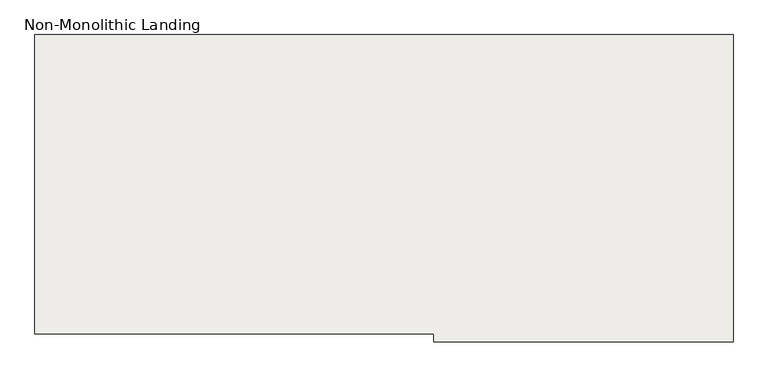
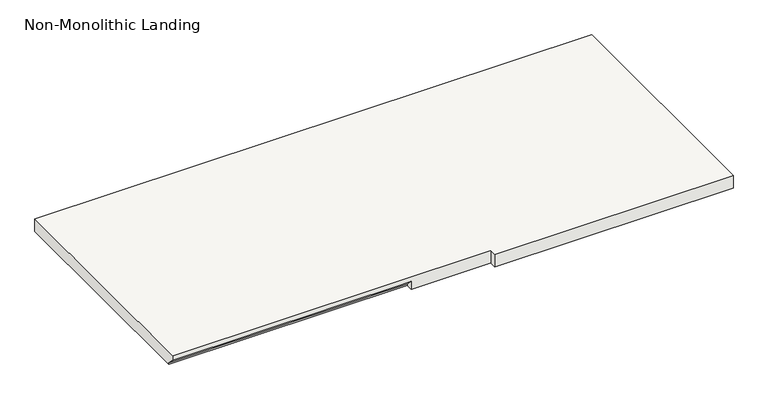
"""IFC4 building model written with IfcOpenShell, lengths in millimetres: slab geometry, Non-Monolithic Landing."""

from ifc_helpers import new_model, si_unit, origin, place, context, project, spatial, faceted_brep, source, transform, mapped, element, save


def non_monolithic_landing_0968bfc6(model_context):
    return source(origin(), model_context, "Body", "Brep", [
        faceted_brep([(-3617.4415084, 23194.7216096, 33512.9005799), (-3617.4415084, 23220.1216096, 33487.5005799), (-2703.0415084, 23220.1216096, 33487.5005799), (-2703.0415084, 23194.7216096, 33512.9005799), (-2398.2415084, 23194.7216096, 33531.9505799), (-2398.2415084, 23169.3216096, 33531.9505799), (-1483.8415084, 23169.3216096, 33531.9505799), (-1483.8415084, 23194.7216096, 33531.9505799), (-1483.8415084, 24109.1216096, 33531.9505799), (-3617.4415084, 24109.1216096, 33531.9505799), (-3617.4415084, 23194.7216096, 33531.9505799), (-2703.0415084, 23220.1216096, 33481.1505799), (-3617.4415084, 23220.1216096, 33481.1505799), (-3617.4415084, 24109.1216096, 33481.1505799), (-1483.8415084, 24109.1216096, 33481.1505799), (-1483.8415084, 23194.7216096, 33481.1505799), (-1483.8415084, 23169.3216096, 33481.1505799), (-2398.2415084, 23169.3216096, 33481.1505799), (-2398.2415084, 23194.7216096, 33481.1505799), (-2703.0415084, 23194.7216096, 33481.1505799)], [[[0, 1, 2, 3]], [[4, 5, 6, 7, 8, 9, 10]], [[11, 12, 13, 14, 15, 16, 17, 18, 19]], [[12, 11, 2, 1]], [[11, 19, 3, 2]], [[4, 10, 0, 3, 19, 18]], [[5, 4, 18, 17]], [[6, 5, 17, 16]], [[7, 6, 16, 15]], [[8, 7, 15, 14]], [[9, 8, 14, 13]], [[10, 9, 13, 12, 1, 0]]]),
    ])


if __name__ == "__main__":
    model = new_model("IFC4")
    model_context = context("Model", 3, world=origin())
    ifc_project = project(units=[si_unit("LENGTHUNIT", "METRE", prefix="MILLI")], contexts=[model_context])
    site = spatial("IfcSite", under=ifc_project)
    building = spatial("IfcBuilding", under=site)
    placement = place(None, origin())
    non_monolithic_landing_shape = non_monolithic_landing_0968bfc6(model_context)
    element("IfcSlab", 1, ObjectType="Non-Monolithic Landing", at=placement, inside=building, context=model_context, shape_type="MappedRepresentation", body=[
        mapped(non_monolithic_landing_shape, transform((0.0, 0.0, 0.0), x_axis=(1.0, 0.0, 0.0), y_axis=(0.0, 1.0, 0.0), z_axis=(0.0, 0.0, 1.0))),
    ])
    save(model, "model.ifc")
